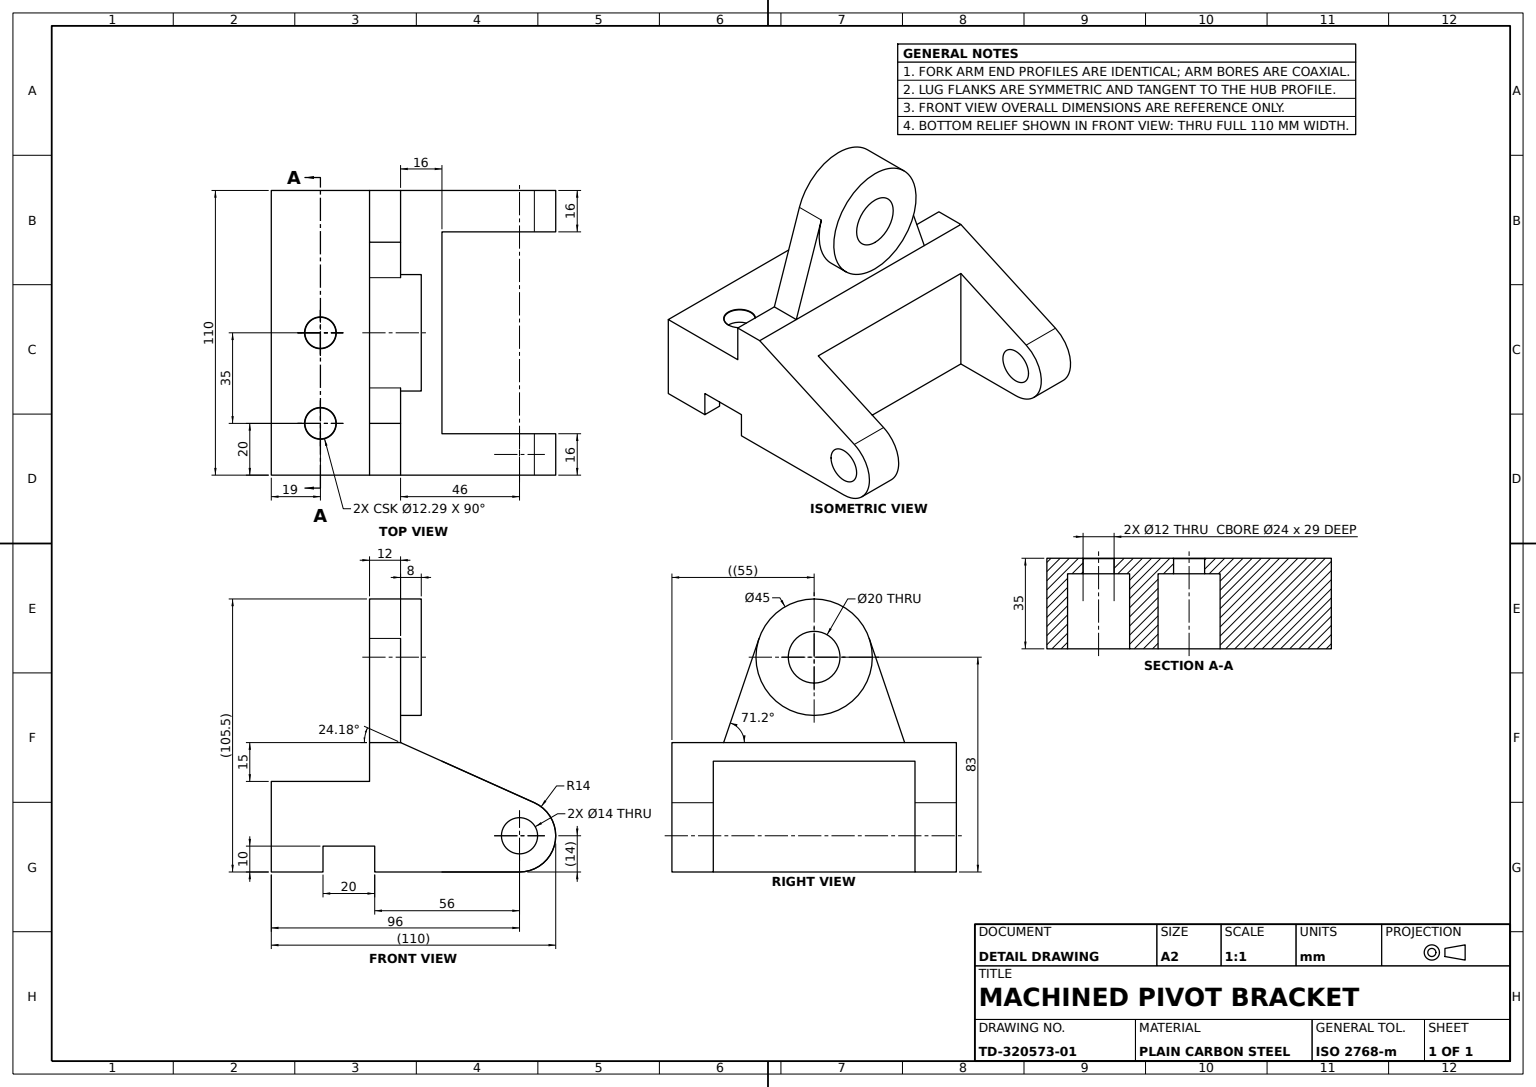
SolidWorks part; units mm, degrees
material "Plain Carbon Steel"
ref_plane "Front Plane" through (0, 0, 0) normal (0, 0, 1) x (1, 0, 0)
ref_plane "Top Plane" through (0, 0, 0) normal (0, 1, 0) x (1, 0, 0)
ref_plane "Right Plane" through (0, 0, 0) normal (1, 0, 0) x (0, 0, -1)
sketch "Base Block Profile Sketch" plane through (0, 0, 0) normal (0, 0, 1) x (1, 0, 0)
  line L0 (-48, 0) -> (48, 0)
  line L1 (48, 0) -> (48, 35)
  line L2 (48, 35) -> (-48, 35)
  line L3 (-48, 35) -> (-48, 0)
  point P4 (0, 0)
  dimension "D1" = 96
  dimension "D2" = 35
  dimension "D3" = 35
extrude "Base Block" add sketch "Base Block Profile Sketch" along normal mid plane 110
sketch "Base Step Recess Sketch" plane through (0, 35, 0) normal (0, 1, 0) x (1, 0, 0)
  line L1 (-48, -55) -> (-48, 55) construction
  line L9 (48, 55) -> (-48, 55) construction
  line L10 (48, -55) -> (-48, -55) construction
  line L11 (47.0035, 55) -> (2, 55)
  line L12 (2, 55) -> (2, -55)
  line L13 (2, -55) -> (48, -55)
  line L14 (48, -55) -> (48, 55)
  dimension "D1" = 110
  dimension "D2" = 46
  dimension "D3" = 95.0035
extrude "Base Step Recess" cut sketch "Base Step Recess Sketch" against normal blind 35 and the other way through all
sketch "Base Groove 20x20 Sketch" plane through (0, 0, 55) normal (0, 0, 1) x (1, 0, 0)
  line L0 (-28, 0) -> (-28, 10)
  line L1 (-48, 0) -> (2, 0) construction
  line L2 (-28, 10) -> (-8, 10)
  line L3 (-8, 10) -> (-8, 0)
  line L4 (-8, 0) -> (-28, 0)
  dimension "D1" = 20
  dimension "D2" = 20
  dimension "D3" = 10
extrude "Base Groove 20x20" cut sketch "Base Groove 20x20 Sketch" against normal blind 110
sketch "Upright Pad Sketch" plane through (0, 35, 0) normal (0, 1, 0) x (1, 0, 0)
  line L0 (2, 55) -> (-10, 55)
  line L1 (2, 55) -> (-48, 55) construction
  line L2 (-10, 55) -> (-10, -55)
  line L3 (2, -55) -> (-48, -55) construction
  line L4 (-10, -55) -> (2, -55)
  line L5 (2, -55) -> (2, 55)
  dimension "D1" = 12
extrude "Upright Pad" add sketch "Upright Pad Sketch" along normal blind 15
sketch "Lug Plate Sketch" plane through (2, 0, 0) normal (1, 0, 0) x (0, 0, -1)
  line L0 (0, 0) -> (0, 83) construction
  line L1 (-35, 50) -> (-21.3, 90.25)
  line L2 (0, 50) -> (-35, 50)
  line L3 (-55, 50) -> (55, 50) construction
  line L4 (0, 50) -> (35, 50)
  line L5 (21.3, 90.25) -> (35, 50)
  arc A1 (21.3, 90.25) -> (-21.3, 90.25) centre (0, 83) ccw
  dimension "D1" = 83
  dimension "D4" = 45
  dimension "D2" = 35
  dimension "D3" = 35
extrude "Lug Plate" add sketch "Lug Plate Sketch" against normal blind 12
sketch "Lug Hub Sketch" plane through (2, 0, 0) normal (1, 0, 0) x (0, 0, -1)
  circle A0 centre (0, 83) radius 22.5
  dimension "D1" = 45
extrude "Lug Hub" add sketch "Lug Hub Sketch" along normal blind 8
sketch "Lug Bore Ø20 Sketch" plane through (10, 0, 0) normal (1, 0, 0) x (0, 0, -1)
  circle A0 centre (0, 83) radius 10
  dimension "D1" = 20
extrude "Lug Bore Ø20" cut sketch "Lug Bore Ø20 Sketch" against normal blind 20
sketch "Side Arm A Sketch" plane through (0, 0, -55) normal (0, 0, -1) x (-1, 0, 0)
  line L0 (8, 0) -> (-48, 0)
  line L1 (-48, 0) -> (-48, 14) construction
  line L2 (-2, 50) -> (-53.7344, 26.7717)
  line L3 (-2, 50) -> (10, 50)
  line L4 (10, 50) -> (10, 35)
  line L5 (10, 35) -> (10, 10)
  line L6 (8, 10) -> (28, 10) construction
  line L7 (10, 10) -> (8, 10)
  line L8 (8, 10) -> (8, 0)
  arc A0 (-53.7344, 26.7717) -> (-48, 0) centre (-48, 14) ccw
  dimension "D1" = 56
  dimension "D2" = 14
extrude "Side Arm A" add sketch "Side Arm A Sketch" against normal blind 16
sketch "Side Arm B Sketch" plane through (0, 0, 55) normal (0, 0, 1) x (1, 0, 0)
  line L0 (-8, 0) -> (48, 0)
  line L1 (48, 0) -> (48, 14) construction
  line L2 (53.7344, 26.7717) -> (2, 50)
  line L3 (2, 50) -> (-10, 50)
  line L4 (-10, 50) -> (-10, 35)
  line L5 (-10, 35) -> (-13.136, 35)
  line L6 (-10, 35) -> (-48, 35) construction
  line L7 (-13.136, 35) -> (-13.136, 10)
  line L8 (-8, 10) -> (-28, 10) construction
  line L9 (-13.136, 10) -> (-8, 10)
  line L10 (-8, 0) -> (-8, 10) construction
  line L11 (-8, 10) -> (-8, 0)
  line L12 (2, 50) -> (2, 0) construction
  arc A0 (48, 0) -> (53.7344, 26.7717) centre (48, 14) ccw
  dimension "D1" = 56
  dimension "D2" = 14
  dimension "D3" = 15.136
extrude "Side Arm B" add sketch "Side Arm B Sketch" against normal blind 16
sketch "Arm B Eye Hole Ø14 Sketch" plane through (0, 0, 55) normal (0, 0, 1) x (1, 0, 0)
  circle A0 centre (48, 14) radius 7
  dimension "D1" = 14
extrude "Arm B Eye Hole Ø14" cut sketch "Arm B Eye Hole Ø14 Sketch" against normal blind 16
sketch "Arm A Eye Hole Ø14 Sketch" plane through (0, 0, -55) normal (0, 0, -1) x (-1, 0, 0)
  circle A0 centre (-48, 14) radius 7
  dimension "D1" = 14
extrude "Arm A Eye Hole Ø14" cut sketch "Arm A Eye Hole Ø14 Sketch" against normal blind 16
sketch "Cross Web Sketch" plane through (0, 50, 0) normal (0, 1, 0) x (1, 0, 0)
  line L0 (2, 39) -> (18, 39)
  line L1 (2, 39) -> (53.7344, 39) construction
  line L2 (18, 39) -> (18, -39)
  line L3 (53.7344, -39) -> (2, -39) construction
  line L4 (18, -39) -> (2, -39)
  line L5 (2, -39) -> (2, 39)
  dimension "D1" = 16
extrude "Cross Web" add sketch "Cross Web Sketch" against normal blind 50
sketch "Triangular Relief Sketch" plane through (0, 0, 39) normal (0, 0, 1) x (1, 0, 0)
  line L0 (2, 50) -> (18, 42.8161)
  line L1 (53.7344, 26.7717) -> (2, 50) construction
  line L2 (18, 42.8161) -> (18, 50) construction
  line L3 (18, 42.8161) -> (18, 50)
  line L4 (2, 50) -> (18, 50) construction
  line L5 (18, 50) -> (2, 50)
extrude "Triangular Relief Cut" cut sketch "Triangular Relief Sketch" against normal up to next
hole_wizard "Counterbored Bolt Hole" positions "Sketch41" profile "Sketch42" counterbore size "M5" standard "ANSI Metric" end condition through all
sketch "Sketch41" plane through (0, 35, 0) normal (0, 1, 0) x (1, 0, 0)
  line L0 (-10, -55) -> (-48, -55) construction
  point P0 (-29, -35)
  point P2 (-29, 0)
  dimension "D1" = 20
  dimension "35" = 35
sketch "Sketch42" plane through (-29, 35, 35) normal (1, 0, 0) x (0, 0, 1)
  line L0 (0, 0) -> (0, 35)
  line L1 (0, 35) -> (12, 35)
  line L3 (12, 35) -> (12, 6)
  line L4 (6, 6) -> (12, 6)
  line L5 (6, 6) -> (6, 0.145)
  line L6 (6, 0.145) -> (6.145, 0)
  line L7 (6.145, 0) -> (0, 0)
  line L8 (-6, 0.145) -> (-6.145, 0) construction
  line L11 (0, -6.35) -> (0, 107.95) construction
  dimension "Thru Hole Dia." = 24
  dimension "Thru Hole Depth" = 35
  dimension "C'Bore Dia." = 12
  dimension "C'Bore Depth" = 6
  dimension "Near C'Sink Dia." = 12.29
  dimension "Near C'Sink Angle" = 90
